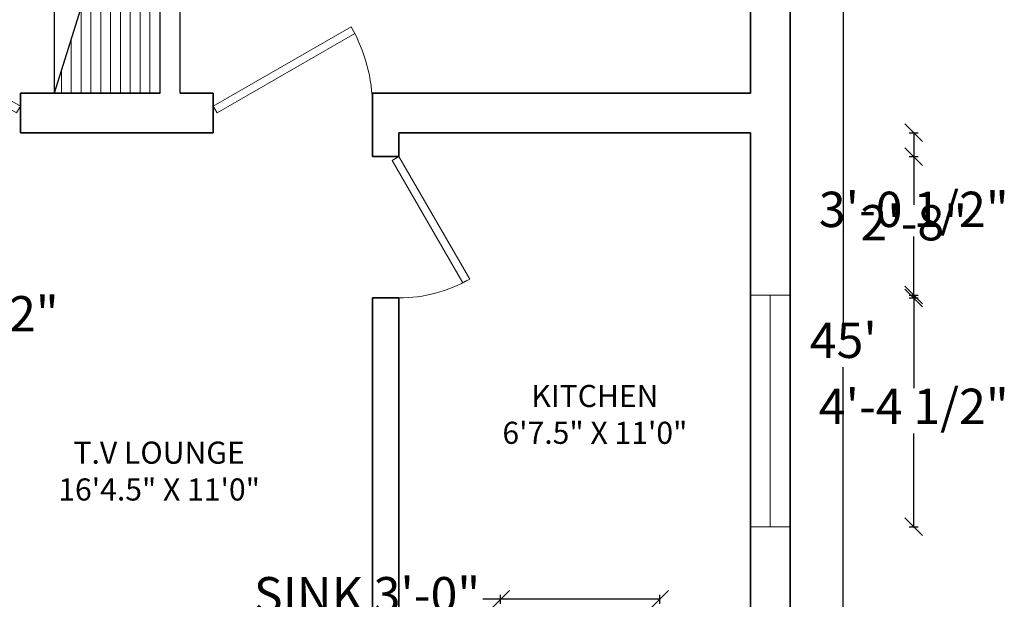
# Model space of a CAD drawing. Units: inches. Extents: x 2558 to 3026, y 433 to 1053.
# Tile 7 of 8: x 2795 to 3018, y 685 to 816. Entities that reach past the tile are written whole.
import ezdxf

# ---------------------------------------------------------------- set-up
doc = ezdxf.new("R2010")
doc.units = ezdxf.units.IN
for name, color, linetype, lineweight in [('A-ANNO-DIMS', 2, 'Continuous', 18), ('A-AREA-IDEN', 7, 'Continuous', 18), ('A-DOOR', 4, 'Continuous', 18), ('A-FLOR-CASE', 8, 'Continuous', 25), ('A-FLOR-CASE-PATT', 8, 'Continuous', 13), ('A-GLAZ', 5, 'Continuous', 18), ('A-WALL', 7, 'Continuous', 35)]:
    doc.layers.add(name, color=color, linetype=linetype, lineweight=lineweight)
doc.styles.get("Standard").update_dxf_attribs({"font": 'arial.ttf'})
doc.dimstyles.new('ISO-25', dxfattribs={"dimtxt": 8, "dimasz": 4, "dimexe": 1, "dimexo": 1, "dimgap": 1, "dimtad": 0, "dimtih": 1, "dimtoh": 1, "dimlunit": 3, "dimtxsty": 'Standard', "dimblk": 'OBLIQUE', "dimcen": 2.5, "dimclrt": 1, "dimadec": 0, "dimazin": 0, "dimtfac": 1, "dimtmove": 0, "dimatfit": 3, "dimfxl": 1, "dimfxlon": 1, "dimarcsym": 0})

# ---------------------------------------------------------------- blocks, each defined once
blk = doc.blocks.new('*U7')
for p, q in [((0, 0), (0, -6)), ((32, 0), (32, -6))]:
    blk.add_line(p, q)
blk.add_lwpolyline([(0, 0), (27.71, 16), (28.59, 14.48), (0.87, -1.52)], close=True)
blk.add_arc((0, 0), 32, 0, 30)
blk = doc.blocks.new('*U9')
for p, q in [((0, 0), (0, -6)), ((-36, 0), (-36, -6))]:
    blk.add_line(p, q)
blk.add_lwpolyline([(0, 0), (-31.18, 18), (-32.05, 16.48), (-0.88, -1.52)], close=True)
blk.add_arc((0, 0), 36, 150, 180)
blk = doc.blocks.new('*U8')
for p, q in [((0, 0), (0, -6)), ((36, 0), (36, -6))]:
    blk.add_line(p, q)
blk.add_lwpolyline([(0, 0), (31.18, 18), (32.05, 16.48), (0.87, -1.52)], close=True)
blk.add_arc((0, 0), 36, 0, 30)
blk = doc.blocks.new('_Oblique')
at = {"color": 0, "linetype": 'ByBlock', "lineweight": -2}
blk.add_line((-0.5, -0.5), (0.5, 0.5), dxfattribs=at)
blk = doc.blocks.new('*D19')
at = {"layer": 'A-ANNO-DIMS', "color": 0, "lineweight": -2, "transparency": 16777216}
for p, q in [((2980.65, 1012.82), (2982.65, 1012.82)), ((2981.65, 1012.82), (2981.65, 747.89)), ((2981.65, 472.82), (2981.65, 737.76)), ((2980.65, 472.82), (2982.65, 472.82))]:
    blk.add_line(p, q, dxfattribs=at)
at = {"layer": 'Defpoints', "color": 0, "transparency": 16777216}
for p in [(2969.63, 1012.82), (2969.63, 472.82), (2981.65, 472.82)]:
    blk.add_point(p, dxfattribs=at)
at = {"layer": 'A-ANNO-DIMS', "color": 0, "lineweight": -2, "transparency": 16777216, "xscale": 4, "yscale": 4, "zscale": 4}
for p, rotation in [((2981.65, 1012.82), 90), ((2981.65, 472.82), 270)]:
    blk.add_blockref('_Oblique', p, dxfattribs=dict(at, rotation=rotation))
at = {"layer": 'A-ANNO-DIMS', "color": 0, "transparency": 16777216, "insert": (2981.65, 742.82), "char_height": 8, "attachment_point": 5}
blk.add_mtext("45'", dxfattribs=at)
blk = doc.blocks.new('*D40')
at = {"layer": 'A-ANNO-DIMS', "color": 0, "lineweight": -2, "transparency": 16777216}
for p, q in [((2733.24, 749.82), (2733.24, 747.82)), ((2733.24, 748.82), (2757.67, 748.82)), ((2757.67, 749.82), (2757.67, 747.82)), ((2757.67, 748.82), (2761.67, 748.82))]:
    blk.add_line(p, q, dxfattribs=at)
at = {"layer": 'Defpoints', "color": 0, "transparency": 16777216}
for p in [(2733.24, 752.87), (2757.67, 752.87), (2757.67, 748.82)]:
    blk.add_point(p, dxfattribs=at)
at = {"layer": 'A-ANNO-DIMS', "color": 0, "lineweight": -2, "transparency": 16777216, "xscale": 4, "yscale": 4, "zscale": 4, "rotation": 180}
blk.add_blockref('_Oblique', (2733.24, 748.82), dxfattribs=at)
at = {"layer": 'A-ANNO-DIMS', "color": 0, "lineweight": -2, "transparency": 16777216, "xscale": 4, "yscale": 4, "zscale": 4}
blk.add_blockref('_Oblique', (2757.67, 748.82), dxfattribs=at)
at = {"layer": 'A-ANNO-DIMS', "color": 1, "transparency": 16777216, "insert": (2782.69, 748.82), "char_height": 8, "attachment_point": 5}
blk.add_mtext('2\'-0 1/2"', dxfattribs=at)
blk = doc.blocks.new('*D41')
at = {"layer": 'A-ANNO-DIMS', "color": 0, "lineweight": -2, "transparency": 16777216}
for p, q in [((2904.13, 684.22), (2904.13, 686.22)), ((2940.13, 684.22), (2940.13, 686.22)), ((2904.13, 685.22), (2900.13, 685.22)), ((2940.13, 685.22), (2904.13, 685.22))]:
    blk.add_line(p, q, dxfattribs=at)
at = {"layer": 'Defpoints', "color": 0, "transparency": 16777216}
for p in [(2904.13, 685.22), (2904.13, 679.82), (2940.13, 679.82)]:
    blk.add_point(p, dxfattribs=at)
at = {"layer": 'A-ANNO-DIMS', "color": 0, "lineweight": -2, "transparency": 16777216, "xscale": 4, "yscale": 4, "zscale": 4, "rotation": 180}
blk.add_blockref('_Oblique', (2904.13, 685.22), dxfattribs=at)
at = {"layer": 'A-ANNO-DIMS', "color": 0, "lineweight": -2, "transparency": 16777216, "xscale": 4, "yscale": 4, "zscale": 4}
blk.add_blockref('_Oblique', (2940.13, 685.22), dxfattribs=at)
at = {"layer": 'A-ANNO-DIMS', "color": 1, "transparency": 16777216, "insert": (2873.92, 685.22), "char_height": 8, "attachment_point": 5}
blk.add_mtext('SINK 3\'-0"', dxfattribs=at)
blk = doc.blocks.new('*D45')
at = {"layer": 'A-ANNO-DIMS', "color": 0, "lineweight": -2, "transparency": 16777216}
for p, q in [((2803.13, 445.87), (2803.13, 443.87)), ((2831.63, 445.87), (2831.63, 443.87)), ((2803.13, 444.87), (2831.63, 444.87)), ((2831.63, 444.87), (2835.63, 444.87))]:
    blk.add_line(p, q, dxfattribs=at)
at = {"layer": 'Defpoints', "color": 0, "transparency": 16777216}
for p in [(2803.13, 799.82), (2831.63, 799.82), (2831.63, 444.87)]:
    blk.add_point(p, dxfattribs=at)
at = {"layer": 'A-ANNO-DIMS', "color": 0, "lineweight": -2, "transparency": 16777216, "xscale": 4, "yscale": 4, "zscale": 4, "rotation": 180}
blk.add_blockref('_Oblique', (2803.13, 444.87), dxfattribs=at)
at = {"layer": 'A-ANNO-DIMS', "color": 0, "lineweight": -2, "transparency": 16777216, "xscale": 4, "yscale": 4, "zscale": 4}
blk.add_blockref('_Oblique', (2831.63, 444.87), dxfattribs=at)
at = {"layer": 'A-ANNO-DIMS', "color": 1, "transparency": 16777216, "insert": (2856.65, 444.87), "char_height": 8, "attachment_point": 5}
blk.add_mtext('2\'-4 1/2"', dxfattribs=at)
blk = doc.blocks.new('*D49')
at = {"layer": 'A-ANNO-DIMS', "color": 0, "lineweight": -2, "transparency": 16777216}
for p, q in [((2839.13, 445.87), (2839.13, 443.87)), ((2875.13, 445.87), (2875.13, 443.87)), ((2839.13, 444.87), (2845.5, 444.87)), ((2875.13, 444.87), (2868.76, 444.87))]:
    blk.add_line(p, q, dxfattribs=at)
at = {"layer": 'Defpoints', "color": 0, "transparency": 16777216}
for p in [(2839.13, 790.82), (2875.13, 790.82), (2875.13, 444.87)]:
    blk.add_point(p, dxfattribs=at)
at = {"layer": 'A-ANNO-DIMS', "color": 0, "lineweight": -2, "transparency": 16777216, "xscale": 4, "yscale": 4, "zscale": 4, "rotation": 180}
blk.add_blockref('_Oblique', (2839.13, 444.87), dxfattribs=at)
at = {"layer": 'A-ANNO-DIMS', "color": 0, "lineweight": -2, "transparency": 16777216, "xscale": 4, "yscale": 4, "zscale": 4}
blk.add_blockref('_Oblique', (2875.13, 444.87), dxfattribs=at)
at = {"layer": 'A-ANNO-DIMS', "color": 1, "transparency": 16777216, "insert": (2857.13, 444.87), "char_height": 8, "attachment_point": 5}
blk.add_mtext('3\'-0"', dxfattribs=at)
blk = doc.blocks.new('*D55')
at = {"layer": 'A-ANNO-DIMS', "color": 0, "lineweight": -2, "transparency": 16777216}
for p, q in [((2996.58, 754.08), (2998.58, 754.08)), ((2997.58, 754.08), (2997.58, 733)), ((2997.58, 701.65), (2997.58, 722.73)), ((2996.58, 701.65), (2998.58, 701.65))]:
    blk.add_line(p, q, dxfattribs=at)
at = {"layer": 'Defpoints', "color": 0, "transparency": 16777216}
for p in [(2969.63, 754.08), (2997.58, 754.08), (2969.63, 701.65)]:
    blk.add_point(p, dxfattribs=at)
at = {"layer": 'A-ANNO-DIMS', "color": 0, "lineweight": -2, "transparency": 16777216, "xscale": 4, "yscale": 4, "zscale": 4}
for p, rotation in [((2997.58, 754.08), 90), ((2997.58, 701.65), 270)]:
    blk.add_blockref('_Oblique', p, dxfattribs=dict(at, rotation=rotation))
at = {"layer": 'A-ANNO-DIMS', "color": 1, "transparency": 16777216, "insert": (2997.58, 727.86), "char_height": 8, "attachment_point": 5}
blk.add_mtext('4\'-4 1/2"', dxfattribs=at)
blk = doc.blocks.new('*D58')
at = {"layer": 'A-ANNO-DIMS', "color": 0, "lineweight": -2, "transparency": 16777216}
for p, q in [((2901.29, 1039.77), (2901.29, 1041.77)), ((2901.29, 1040.77), (2910.69, 1040.77)), ((2943.34, 1040.77), (2933.95, 1040.77)), ((2943.34, 1039.77), (2943.34, 1041.77))]:
    blk.add_line(p, q, dxfattribs=at)
at = {"layer": 'Defpoints', "color": 0, "transparency": 16777216}
for p in [(2943.34, 1040.77), (2901.29, 649.82), (2943.34, 649.82)]:
    blk.add_point(p, dxfattribs=at)
at = {"layer": 'A-ANNO-DIMS', "color": 0, "lineweight": -2, "transparency": 16777216, "xscale": 4, "yscale": 4, "zscale": 4, "rotation": 180}
blk.add_blockref('_Oblique', (2901.29, 1040.77), dxfattribs=at)
at = {"layer": 'A-ANNO-DIMS', "color": 0, "lineweight": -2, "transparency": 16777216, "xscale": 4, "yscale": 4, "zscale": 4}
blk.add_blockref('_Oblique', (2943.34, 1040.77), dxfattribs=at)
at = {"layer": 'A-ANNO-DIMS', "color": 1, "transparency": 16777216, "insert": (2922.32, 1040.77), "char_height": 8, "attachment_point": 5}
blk.add_mtext('3\'-6"', dxfattribs=at)
blk = doc.blocks.new('*D63')
at = {"layer": 'A-ANNO-DIMS', "color": 0, "lineweight": -2, "transparency": 16777216}
for p, q in [((2757.89, 445.87), (2757.89, 443.87)), ((2765.63, 445.87), (2765.63, 443.87)), ((2757.89, 444.87), (2765.63, 444.87)), ((2765.63, 444.87), (2769.63, 444.87))]:
    blk.add_line(p, q, dxfattribs=at)
at = {"layer": 'Defpoints', "color": 0, "transparency": 16777216}
for p in [(2757.89, 943.82), (2765.63, 943.82), (2765.63, 444.87)]:
    blk.add_point(p, dxfattribs=at)
at = {"layer": 'A-ANNO-DIMS', "color": 0, "lineweight": -2, "transparency": 16777216, "xscale": 4, "yscale": 4, "zscale": 4, "rotation": 180}
blk.add_blockref('_Oblique', (2757.89, 444.87), dxfattribs=at)
at = {"layer": 'A-ANNO-DIMS', "color": 0, "lineweight": -2, "transparency": 16777216, "xscale": 4, "yscale": 4, "zscale": 4}
blk.add_blockref('_Oblique', (2765.63, 444.87), dxfattribs=at)
at = {"layer": 'A-ANNO-DIMS', "color": 1, "transparency": 16777216, "insert": (2790.59, 444.87), "char_height": 8, "attachment_point": 5}
blk.add_mtext('0\'-7 1/2"', dxfattribs=at)
blk = doc.blocks.new('*D67')
at = {"layer": 'A-ANNO-DIMS', "color": 0, "lineweight": -2, "transparency": 16777216}
for p, q in [((2996.58, 790.82), (2998.58, 790.82)), ((2997.58, 790.82), (2997.58, 777.59)), ((2997.58, 754.08), (2997.58, 767.31)), ((2996.58, 754.08), (2998.58, 754.08))]:
    blk.add_line(p, q, dxfattribs=at)
at = {"layer": 'Defpoints', "color": 0, "transparency": 16777216}
for p in [(2960.63, 790.82), (2997.58, 790.82), (2969.63, 754.08)]:
    blk.add_point(p, dxfattribs=at)
at = {"layer": 'A-ANNO-DIMS', "color": 0, "lineweight": -2, "transparency": 16777216, "xscale": 4, "yscale": 4, "zscale": 4}
for p, rotation in [((2997.58, 790.82), 90), ((2997.58, 754.08), 270)]:
    blk.add_blockref('_Oblique', p, dxfattribs=dict(at, rotation=rotation))
at = {"layer": 'A-ANNO-DIMS', "color": 1, "transparency": 16777216, "insert": (2997.58, 772.45), "char_height": 8, "attachment_point": 5}
blk.add_mtext('3\'-0 1/2"', dxfattribs=at)
blk = doc.blocks.new('*D72')
at = {"layer": 'A-ANNO-DIMS', "color": 0, "lineweight": -2, "transparency": 16777216}
for p, q in [((2996.58, 785.43), (2998.58, 785.43)), ((2997.58, 785.43), (2997.58, 774.52)), ((2997.58, 753.43), (2997.58, 764.35)), ((2996.58, 753.43), (2998.58, 753.43))]:
    blk.add_line(p, q, dxfattribs=at)
at = {"layer": 'Defpoints', "color": 0, "transparency": 16777216}
for p in [(2881.13, 785.43), (2997.58, 785.43), (2881.13, 753.43)]:
    blk.add_point(p, dxfattribs=at)
at = {"layer": 'A-ANNO-DIMS', "color": 0, "lineweight": -2, "transparency": 16777216, "xscale": 4, "yscale": 4, "zscale": 4}
for p, rotation in [((2997.58, 785.43), 90), ((2997.58, 753.43), 270)]:
    blk.add_blockref('_Oblique', p, dxfattribs=dict(at, rotation=rotation))
at = {"layer": 'A-ANNO-DIMS', "color": 1, "transparency": 16777216, "insert": (2997.58, 769.43), "char_height": 8, "attachment_point": 5}
blk.add_mtext('2\'-8"', dxfattribs=at)
blk = doc.blocks.new('*D73')
at = {"layer": 'A-ANNO-DIMS', "color": 0, "lineweight": -2, "transparency": 16777216}
for p, q in [((2816.63, 1039.77), (2816.63, 1041.77)), ((2816.63, 1040.77), (2870.66, 1040.77)), ((2959.63, 1040.77), (2905.6, 1040.77)), ((2959.63, 1039.77), (2959.63, 1041.77))]:
    blk.add_line(p, q, dxfattribs=at)
at = {"layer": 'Defpoints', "color": 0, "transparency": 16777216}
for p in [(2959.63, 1040.77), (2816.63, 481.83), (2959.63, 481.82)]:
    blk.add_point(p, dxfattribs=at)
at = {"layer": 'A-ANNO-DIMS', "color": 0, "lineweight": -2, "transparency": 16777216, "xscale": 4, "yscale": 4, "zscale": 4, "rotation": 180}
blk.add_blockref('_Oblique', (2816.63, 1040.77), dxfattribs=at)
at = {"layer": 'A-ANNO-DIMS', "color": 0, "lineweight": -2, "transparency": 16777216, "xscale": 4, "yscale": 4, "zscale": 4}
blk.add_blockref('_Oblique', (2959.63, 1040.77), dxfattribs=at)
at = {"layer": 'A-ANNO-DIMS', "color": 1, "transparency": 16777216, "insert": (2888.13, 1040.77), "char_height": 8, "attachment_point": 5}
blk.add_mtext('11\'-11"', dxfattribs=at)
blk = doc.blocks.new('*D75')
at = {"layer": 'A-ANNO-DIMS', "color": 0, "lineweight": -2, "transparency": 16777216}
for p, q in [((2831.63, 445.87), (2831.63, 443.87)), ((2839.13, 445.87), (2839.13, 443.87)), ((2831.63, 444.87), (2839.13, 444.87)), ((2839.13, 444.87), (2843.13, 444.87))]:
    blk.add_line(p, q, dxfattribs=at)
at = {"layer": 'Defpoints', "color": 0, "transparency": 16777216}
for p in [(2831.63, 799.82), (2839.13, 799.82), (2839.13, 444.87)]:
    blk.add_point(p, dxfattribs=at)
at = {"layer": 'A-ANNO-DIMS', "color": 0, "lineweight": -2, "transparency": 16777216, "xscale": 4, "yscale": 4, "zscale": 4, "rotation": 180}
blk.add_blockref('_Oblique', (2831.63, 444.87), dxfattribs=at)
at = {"layer": 'A-ANNO-DIMS', "color": 0, "lineweight": -2, "transparency": 16777216, "xscale": 4, "yscale": 4, "zscale": 4}
blk.add_blockref('_Oblique', (2839.13, 444.87), dxfattribs=at)
at = {"layer": 'A-ANNO-DIMS', "color": 1, "transparency": 16777216, "insert": (2864.09, 444.87), "char_height": 8, "attachment_point": 5}
blk.add_mtext('0\'-7 1/2"', dxfattribs=at)
blk = doc.blocks.new('*D76')
at = {"layer": 'A-ANNO-DIMS', "color": 0, "lineweight": -2, "transparency": 16777216}
for p, q in [((2879.03, 445.87), (2879.03, 443.87)), ((2911.03, 445.87), (2911.03, 443.87)), ((2879.03, 444.87), (2883.32, 444.87)), ((2911.03, 444.87), (2906.73, 444.87))]:
    blk.add_line(p, q, dxfattribs=at)
at = {"layer": 'Defpoints', "color": 0, "transparency": 16777216}
for p in [(2879.03, 943.82), (2911.03, 943.82), (2911.03, 444.87)]:
    blk.add_point(p, dxfattribs=at)
at = {"layer": 'A-ANNO-DIMS', "color": 0, "lineweight": -2, "transparency": 16777216, "xscale": 4, "yscale": 4, "zscale": 4, "rotation": 180}
blk.add_blockref('_Oblique', (2879.03, 444.87), dxfattribs=at)
at = {"layer": 'A-ANNO-DIMS', "color": 0, "lineweight": -2, "transparency": 16777216, "xscale": 4, "yscale": 4, "zscale": 4}
blk.add_blockref('_Oblique', (2911.03, 444.87), dxfattribs=at)
at = {"layer": 'A-ANNO-DIMS', "color": 1, "transparency": 16777216, "insert": (2895.03, 444.87), "char_height": 8, "attachment_point": 5}
blk.add_mtext('2\'-8"', dxfattribs=at)

msp = doc.modelspace()

# ---------------------------------------------------------------- hatches: boundary and pattern name
at = {"layer": 'A-FLOR-CASE-PATT'}
h = msp.add_hatch(dxfattribs=at)
h.set_pattern_fill('ANSI31', color=256, scale=0.7, angle=45)
h.set_pattern_definition([(90, (0, 4.5), (-2.2225, 0), [])])
h.paths.add_polyline_path([(2831.633, 943.825), (2807.633, 943.825), (2807.633, 876.325)])
h.paths.add_polyline_path([(2827.133, 876.325), (2803.133, 799.825), (2827.133, 799.825)])

# ---------------------------------------------------------------- linework, layer by layer
at = {"layer": 'A-FLOR-CASE'}
for p, q in [((2803.133, 952.825), (2803.133, 799.825)), ((2831.633, 799.825), (2831.633, 952.825)), ((2827.133, 876.325), (2803.133, 799.825)), ((2827.133, 799.825), (2827.133, 876.325))]:
    msp.add_line(p, q, dxfattribs=at)
at = {"layer": 'A-GLAZ'}
for p, q in [((2960.633, 754.077), (2969.633, 754.077)), ((2965.133, 754.077), (2965.133, 701.648)), ((2960.633, 701.648), (2969.633, 701.648))]:
    msp.add_line(p, q, dxfattribs=at)
at = {"layer": 'A-WALL'}
for p, q in [((2969.633, 472.825), (2969.633, 1012.825)), ((2960.633, 799.825), (2960.633, 943.825)), ((2795.497, 799.825), (2795.497, 790.825)), ((2827.133, 799.825), (2795.497, 799.825)), ((2839.133, 799.825), (2831.633, 799.825)), ((2839.133, 799.825), (2839.133, 790.825)), ((2960.633, 799.825), (2875.133, 799.825)), ((2875.133, 799.825), (2875.133, 785.433)), ((2839.133, 790.825), (2795.497, 790.825)), ((2960.633, 790.825), (2881.133, 790.825)), ((2881.133, 785.433), (2881.133, 790.825)), ((2960.633, 658.825), (2960.633, 790.825)), ((2881.133, 785.433), (2875.133, 785.433)), ((2881.133, 753.433), (2875.133, 753.433)), ((2875.133, 753.433), (2875.133, 658.825)), ((2881.133, 658.825), (2881.133, 753.433))]:
    msp.add_line(p, q, dxfattribs=at)

# ---------------------------------------------------------------- block references
at = {"layer": 'A-DOOR'}
for name, p in [('*U9', (2795.497, 796.825)), ('*U8', (2839.133, 796.825))]:
    msp.add_blockref(name, p, dxfattribs=at)
at = {"layer": 'A-DOOR', "rotation": 270}
msp.add_blockref('*U7', (2881.133, 785.433), dxfattribs=at)

# ---------------------------------------------------------------- texts
at = {"layer": 'A-AREA-IDEN', "char_height": 5, "attachment_point": 1}
for s, insert in [('\\pxqc;KITCHEN\\P6\'7.5" X 11\'0"', (2902.425, 733.744)), ('\\pxqc;T.V LOUNGE\\P16\'4.5" X 11\'0"', (2803.856, 720.915))]:
    msp.add_mtext_dynamic_manual_height_columns(s, width=46.06135, gutter_width=12.5, heights=[0], dxfattribs=dict(at, insert=insert))

# ---------------------------------------------------------------- dimensions: what is measured, and where the dimension line sits
at = {"layer": 'A-ANNO-DIMS'}
for base, p1, p2, picture, middle in [((2959.633, 1040.775), (2816.633, 481.827), (2959.633, 481.825), '*D73', (2888.133, 1040.775)), ((2943.3439, 1040.7746), (2901.2944, 649.8246), (2943.3439, 649.8246), '*D58', (2922.3191, 1040.7746)), ((2765.633, 444.875), (2757.892, 943.825), (2765.633, 943.825), '*D63', (2790.586, 444.875)), ((2911.025, 444.875), (2879.025, 943.825), (2911.025, 943.825), '*D76', (2895.025, 444.875)), ((2831.633, 444.875), (2803.133, 799.825), (2831.633, 799.825), '*D45', (2856.654, 444.875)), ((2839.133, 444.875), (2831.633, 799.825), (2839.133, 799.825), '*D75', (2864.086, 444.875)), ((2875.133, 444.875), (2839.133, 790.825), (2875.133, 790.825), '*D49', (2857.133, 444.875)), ((2757.67, 748.821), (2733.235, 752.871), (2757.67, 752.871), '*D40', (2782.692, 748.821))]:
    dim = msp.add_linear_dim(base=base, p1=p1, p2=p2, dimstyle='ISO-25', override={"dimdec": 1, "dimlfac": 1, "dimrnd": 0, "dimzin": 1, "dimdsep": 46, "dimlunit": 4, "dimfrac": 2}, dxfattribs=at)
    dim.commit()
    dim.dimension.update_dxf_attribs({"geometry": picture, "text_midpoint": middle})
for base, p1, p2, override, picture, middle in [((2981.646, 472.825), (2969.633, 1012.825), (2969.633, 472.825), {"dimclrd": 0, "dimclre": 0, "dimclrt": 0}, '*D19', (2981.646, 742.825)), ((2997.583, 790.825), (2969.633, 754.077), (2960.633, 790.825), {"dimdec": 1, "dimlfac": 1, "dimrnd": 0, "dimzin": 1, "dimdsep": 46, "dimlunit": 4, "dimfrac": 2}, '*D67', (2997.583, 772.451)), ((2997.583, 785.433), (2881.133, 753.433), (2881.133, 785.433), {"dimdec": 1, "dimlfac": 1, "dimrnd": 0, "dimzin": 1, "dimdsep": 46, "dimlunit": 4, "dimfrac": 2}, '*D72', (2997.583, 769.433)), ((2997.583, 754.077), (2969.633, 701.648), (2969.633, 754.077), {"dimdec": 1, "dimlfac": 1, "dimrnd": 0, "dimzin": 1, "dimdsep": 46, "dimlunit": 4, "dimfrac": 2}, '*D55', (2997.583, 727.862))]:
    dim = msp.add_linear_dim(base=base, p1=p1, p2=p2, angle=90, dimstyle='ISO-25', override=override, dxfattribs=at)
    dim.commit()
    dim.dimension.update_dxf_attribs({"geometry": picture, "text_midpoint": middle})
dim = msp.add_linear_dim(base=(2904.13, 685.225), p1=(2940.13, 679.825), p2=(2904.13, 679.825), angle=180, text='SINK <>', dimstyle='ISO-25', override={"dimdec": 1, "dimlfac": 1, "dimrnd": 0, "dimzin": 1, "dimdsep": 46, "dimlunit": 4, "dimfrac": 2}, dxfattribs=at)
dim.commit()
dim.dimension.update_dxf_attribs({"geometry": '*D41', "text_midpoint": (2873.922, 685.225)})

doc.saveas('drawing.dxf')
